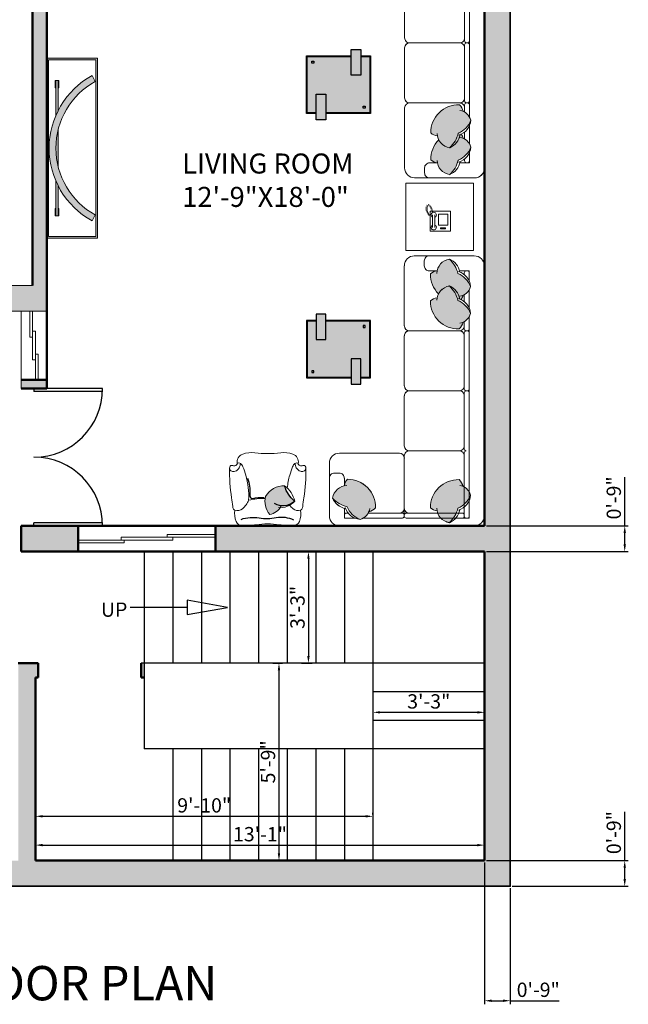
# Model space of a CAD drawing. Units: inches. Extents: x 1734 to 4011, y 1071 to 1891.
# Tile 15 of 27: x 3304 to 3517, y 1071 to 1415. Entities that reach past the tile are written whole.
import ezdxf

# ---------------------------------------------------------------- set-up
doc = ezdxf.new("R2010")
doc.units = ezdxf.units.IN
for name, color, linetype, lineweight in [('A-ANNO-DIMS', 2, 'Continuous', 18), ('A-ANNO-TEXT', 7, 'Continuous', 25), ('A-AREA-IDEN', 3, 'Continuous', 18), ('A-DOOR', 3, 'Continuous', 25), ('A-FLOR-STRS', 2, 'Continuous', 25), ('A-FURN', 8, 'Continuous', 18), ('A-FURN-PATT', 252, 'Continuous', 13), ('A-GLAZ', 4, 'Continuous', 18), ('A-WALL', 7, 'Continuous', 50), ('A-WALL-PATT', 8, 'Continuous', 13), ('aparador', 36, 'Continuous', 9), ('C-PROP', 1, 'Continuous', 35), ('moveis', 254, 'Continuous', 5)]:
    doc.layers.add(name, color=color, linetype=linetype, lineweight=lineweight)
doc.layers.add('IFF-FURN-DETAIL', color=250, linetype='Continuous')
doc.layers.add('MOBIL', color=7, linetype='Continuous')
doc.styles.get("Standard").update_dxf_attribs({"font": 'arial.ttf'})
doc.dimstyles.new('ISO-25', dxfattribs={"dimtxt": 5, "dimasz": 2.5, "dimexe": 1.25, "dimexo": 0.625, "dimtad": 1, "dimdec": 1, "dimlunit": 3, "dimtxsty": 'Standard', "dimcen": 2.5, "dimclrt": 1, "dimadec": 0, "dimazin": 0, "dimtfac": 1, "dimtdec": 1, "dimtmove": 0, "dimatfit": 3, "dimfxl": 1, "dimarcsym": 0})

# ---------------------------------------------------------------- blocks, each defined once
blk = doc.blocks.new('*D62')
at = {"layer": 'A-ANNO-DIMS', "color": 0, "lineweight": -2, "transparency": 16777216}
for p, q in [((3403.06, 1228.82), (3406.68, 1228.82)), ((3405.43, 1226.32), (3405.43, 1192.32)), ((3403.06, 1189.82), (3406.68, 1189.82))]:
    blk.add_line(p, q, dxfattribs=at)
at = {"layer": 'A-ANNO-DIMS', "color": 0, "transparency": 16777216}
for points in [[(3405.01, 1226.32), (3405.85, 1226.32), (3405.43, 1228.82)], [(3405.01, 1192.32), (3405.85, 1192.32), (3405.43, 1189.82)]]:
    blk.add_solid(points, dxfattribs=at)
at = {"layer": 'Defpoints', "color": 0, "transparency": 16777216}
for p in [(3402.43, 1228.82), (3402.43, 1189.82), (3405.43, 1189.82)]:
    blk.add_point(p, dxfattribs=at)
at = {"layer": 'A-ANNO-DIMS', "color": 0, "transparency": 16777216, "insert": (3402.25, 1209.32), "char_height": 5, "attachment_point": 5, "rotation": 90}
blk.add_mtext('3\'-3"', dxfattribs=at)
blk = doc.blocks.new('*D63')
at = {"layer": 'A-ANNO-DIMS', "color": 0, "lineweight": -2, "transparency": 16777216}
for p, q in [((3392.99, 1189.82), (3396.38, 1189.82)), ((3395.13, 1187.32), (3395.13, 1123.32)), ((3392.99, 1120.82), (3396.38, 1120.82))]:
    blk.add_line(p, q, dxfattribs=at)
at = {"layer": 'A-ANNO-DIMS', "color": 0, "transparency": 16777216}
for points in [[(3394.71, 1187.32), (3395.55, 1187.32), (3395.13, 1189.82)], [(3394.71, 1123.32), (3395.55, 1123.32), (3395.13, 1120.82)]]:
    blk.add_solid(points, dxfattribs=at)
at = {"layer": 'Defpoints', "color": 0, "transparency": 16777216}
for p in [(3392.36, 1189.82), (3392.36, 1120.82), (3395.13, 1120.82)]:
    blk.add_point(p, dxfattribs=at)
at = {"layer": 'A-ANNO-DIMS', "color": 0, "transparency": 16777216, "insert": (3391.95, 1155.32), "char_height": 5, "attachment_point": 5, "rotation": 90}
blk.add_mtext('5\'-9"', dxfattribs=at)
blk = doc.blocks.new('*D64')
at = {"layer": 'A-ANNO-DIMS', "color": 0, "lineweight": -2, "transparency": 16777216}
for p, q in [((3309.99, 1136.91), (3309.99, 1137.53)), ((3312.49, 1136.28), (3425.49, 1136.28)), ((3427.99, 1136.91), (3427.99, 1137.53))]:
    blk.add_line(p, q, dxfattribs=at)
at = {"layer": 'A-ANNO-DIMS', "color": 0, "transparency": 16777216}
for points in [[(3312.49, 1136.7), (3312.49, 1135.87), (3309.99, 1136.28)], [(3425.49, 1136.7), (3425.49, 1135.87), (3427.99, 1136.28)]]:
    blk.add_solid(points, dxfattribs=at)
at = {"layer": 'Defpoints', "color": 0, "transparency": 16777216}
for p in [(3309.99, 1136.28), (3427.99, 1136.28), (3427.99, 1136.28)]:
    blk.add_point(p, dxfattribs=at)
at = {"layer": 'A-ANNO-DIMS', "color": 0, "transparency": 16777216, "insert": (3368.99, 1139.46), "char_height": 5, "attachment_point": 5}
blk.add_mtext('9\'-10"', dxfattribs=at)
blk = doc.blocks.new('*D68')
at = {"layer": 'A-ANNO-DIMS', "color": 0, "lineweight": -2, "transparency": 16777216}
for p, q in [((3309.99, 1121.44), (3309.99, 1127.46)), ((3312.49, 1126.21), (3464.49, 1126.21)), ((3466.99, 1121.44), (3466.99, 1127.46))]:
    blk.add_line(p, q, dxfattribs=at)
at = {"layer": 'A-ANNO-DIMS', "color": 0, "transparency": 16777216}
for points in [[(3312.49, 1126.63), (3312.49, 1125.79), (3309.99, 1126.21)], [(3464.49, 1126.63), (3464.49, 1125.79), (3466.99, 1126.21)]]:
    blk.add_solid(points, dxfattribs=at)
at = {"layer": 'Defpoints', "color": 0, "transparency": 16777216}
for p in [(3466.99, 1126.21), (3309.99, 1120.82), (3466.99, 1120.82)]:
    blk.add_point(p, dxfattribs=at)
at = {"layer": 'A-ANNO-DIMS', "color": 0, "transparency": 16777216, "insert": (3388.49, 1129.39), "char_height": 5, "attachment_point": 5}
blk.add_mtext('13\'-1"', dxfattribs=at)
blk = doc.blocks.new('*D69')
at = {"layer": 'A-ANNO-DIMS', "color": 0, "lineweight": -2, "transparency": 16777216}
for p, q in [((3427.99, 1174.19), (3427.99, 1171.38)), ((3466.99, 1173.25), (3466.99, 1173.88)), ((3430.49, 1172.63), (3464.49, 1172.63))]:
    blk.add_line(p, q, dxfattribs=at)
at = {"layer": 'A-ANNO-DIMS', "color": 0, "transparency": 16777216}
for points in [[(3430.49, 1173.04), (3430.49, 1172.21), (3427.99, 1172.63)], [(3464.49, 1173.04), (3464.49, 1172.21), (3466.99, 1172.63)]]:
    blk.add_solid(points, dxfattribs=at)
at = {"layer": 'Defpoints', "color": 0, "transparency": 16777216}
for p in [(3427.99, 1174.82), (3466.99, 1172.63), (3466.99, 1172.63)]:
    blk.add_point(p, dxfattribs=at)
at = {"layer": 'A-ANNO-DIMS', "color": 0, "transparency": 16777216, "insert": (3447.49, 1175.8), "char_height": 5, "attachment_point": 5}
blk.add_mtext('3\'-3"', dxfattribs=at)
blk = doc.blocks.new("MD D 4'")
for p, q in [((0, 24), (0, 0)), ((1, 24), (1, 0)), ((47, 24), (47, 0)), ((48, 24), (48, 0)), ((0, 0), (1, 0)), ((48, 0), (47, 0))]:
    blk.add_line(p, q)
for centre, start, end in [((0, 0), 0, 90), ((48, 0), 90, 180)]:
    blk.add_arc(centre, 24, start, end)
blk = doc.blocks.new('Aparador ORGANICA Formatto')
at = {"layer": 'aparador', "ltscale": 0.3}
h = blk.add_hatch(color=256, dxfattribs=at)
h.dxf.hatch_style = 1
h.set_gradient(color1=(118, 213, 123), color2=(52, 168, 57), one_color=1, tint=0.43, name='INVCURVED')
h.paths.add_polyline_path([(0.8, 0.45), (-0.8, 0.45), (-0.8, 0), (0.8, 0)])
h.paths.add_polyline_path([(0.785, 0.435), (0.785, 0.015), (-0.785, 0.015), (-0.785, 0.435)], flags=16)
h.paths.add_polyline_path([(0.2911, 0.3699), (0.5365, 0.3699), (0.5365, 0.3757), (0.6011, 0.3757), (0.6011, 0.3699), (0.6011, 0.3499), (0.6011, 0.3441), (0.5365, 0.3441), (0.5365, 0.3499), (0.3338, 0.3499, -0.150336), (0.6449, 0.0488), (0.5923, 0.0199, 0.208852), (0.1632, 0.3499), (-0.1632, 0.3499, 0.208852), (-0.5923, 0.0199), (-0.6449, 0.0488, -0.150336), (-0.3338, 0.3499), (-0.5365, 0.3499), (-0.5365, 0.3441), (-0.6011, 0.3441), (-0.6011, 0.3499), (-0.6011, 0.3699), (-0.6011, 0.3757), (-0.5365, 0.3757), (-0.5365, 0.3699), (-0.2911, 0.3699, -0.206106)], flags=0)
h = blk.add_hatch(color=256, dxfattribs=at)
h.dxf.hatch_style = 1
h.set_gradient(color1=(135, 92, 69), color2=(0, 0, 0), one_color=1, name='INVCURVED')
h.paths.add_polyline_path([(-0.6449, 0.0488), (-0.5923, 0.0199, -0.590888), (0.5923, 0.0199), (0.6449, 0.0488, 0.590888)])
h = blk.add_hatch(color=256, dxfattribs=at)
h.dxf.hatch_style = 1
h.set_gradient(color1=(178, 189, 189), one_color=1, tint=1, name='CYLINDER')
h.paths.add_polyline_path([(-0.5365, 0.3757), (-0.6011, 0.3757), (-0.6011, 0.3699), (-0.5365, 0.3699)])
h.paths.add_polyline_path([(-0.5365, 0.3499), (-0.6011, 0.3499), (-0.6011, 0.3441), (-0.5365, 0.3441)])
h = blk.add_hatch(color=256, dxfattribs=at)
h.dxf.hatch_style = 1
h.set_gradient(color1=(118, 213, 123), color2=(31, 101, 35), one_color=1, tint=0.26, name='INVCURVED')
h.paths.add_polyline_path([(-0.2911, 0.3699), (-0.6011, 0.3699), (-0.6011, 0.3499), (-0.3338, 0.3499, -0.015999)])
h = blk.add_hatch(color=256, dxfattribs=at)
h.dxf.hatch_style = 1
h.set_gradient(color1=(118, 213, 123), color2=(31, 101, 35), one_color=1, tint=0.26, name='INVCURVED')
h.paths.add_polyline_path([(-0.1632, 0.3499), (0.1632, 0.3499, 0.122516)])
h = blk.add_hatch(color=256, dxfattribs=at)
h.dxf.hatch_style = 1
h.set_gradient(color1=(118, 213, 123), color2=(31, 101, 35), one_color=1, tint=0.26, name='INVCURVED')
h.paths.add_polyline_path([(0.6011, 0.3699), (0.2911, 0.3699, -0.015999), (0.3338, 0.3499), (0.6011, 0.3499)])
h = blk.add_hatch(color=256, dxfattribs=at)
h.dxf.hatch_style = 1
h.set_gradient(color1=(178, 189, 189), one_color=1, tint=1, name='CYLINDER')
h.paths.add_polyline_path([(0.6011, 0.3757), (0.5365, 0.3757), (0.5365, 0.3699), (0.6011, 0.3699)])
h.paths.add_polyline_path([(0.6011, 0.3499), (0.5365, 0.3499), (0.5365, 0.3441), (0.6011, 0.3441)])
for p, q in [((-0.5923, 0.0199), (-0.6449, 0.0488)), ((0.5923, 0.0199), (0.6449, 0.0488))]:
    blk.add_line(p, q, dxfattribs=at)
for points in [[(-0.6011, 0.3699), (-0.6011, 0.3757), (-0.5365, 0.3757), (-0.5365, 0.3699)], [(-0.5365, 0.3499), (-0.5365, 0.3441), (-0.6011, 0.3441), (-0.6011, 0.3499)], [(0.6011, 0.3699), (0.6011, 0.3757), (0.5365, 0.3757), (0.5365, 0.3699)], [(0.5365, 0.3499), (0.5365, 0.3441), (0.6011, 0.3441), (0.6011, 0.3499)]]:
    blk.add_lwpolyline(points, dxfattribs=at)
for radius in [0.7362, 0.6762]:
    blk.add_arc((0, -0.3063), radius, 28.84335, 151.15665, dxfattribs=at)
at = {"layer": 'moveis', "ltscale": 0.3}
for p, q in [((-0.6011, 0.3699), (-0.6011, 0.3499)), ((-0.2911, 0.3699), (-0.6011, 0.3699)), ((-0.6011, 0.3499), (-0.3338, 0.3499)), ((-0.1632, 0.3499), (0.1632, 0.3499)), ((0.2911, 0.3699), (0.6011, 0.3699)), ((0.6011, 0.3499), (0.3338, 0.3499)), ((0.6011, 0.3699), (0.6011, 0.3499))]:
    blk.add_line(p, q, dxfattribs=at)
for points in [[(-0.8, 0), (0.8, 0), (0.8, 0.45), (-0.8, 0.45)], [(-0.785, 0.015), (0.785, 0.015), (0.785, 0.435), (-0.785, 0.435)]]:
    blk.add_lwpolyline(points, close=True, dxfattribs=at)
blk = doc.blocks.new('Mesa de centro Cantria feeling')
at = {"layer": 'MOBIL', "ltscale": 0.2}
h = blk.add_hatch(color=256, dxfattribs=at)
h.set_gradient(color1=(74, 55, 38), color2=(104, 77, 54), one_color=1, tint=0.31, name='CYLINDER')
h.paths.add_polyline_path([(-0.85, -0.3), (-0.7, -0.3), (-0.7, 0.1), (-0.85, 0.1)])
h = blk.add_hatch(color=256, dxfattribs=at)
h.set_gradient(color1=(221, 221, 223), one_color=1, tint=1)
h.paths.add_polyline_path([(-0.15, -0.6), (-0.15, -0.89), (-0.01, -0.89), (-0.01, -0.01), (-0.7, -0.01), (-0.7, -0.3), (-0.85, -0.3), (-0.85, -0.01), (-0.99, -0.01), (-0.99, -0.89), (-0.3, -0.89), (-0.3, -0.6)])
h.paths.add_polyline_path([(-0.112, -0.112), (-0.112, -0.082), (-0.082, -0.082), (-0.082, -0.112)], flags=16)
h.paths.add_polyline_path([(-0.888, -0.788), (-0.888, -0.818), (-0.918, -0.818), (-0.918, -0.788)], flags=16)
h = blk.add_hatch(color=256, dxfattribs=at)
h.set_gradient(color1=(74, 55, 38), color2=(104, 77, 54), one_color=1, tint=0.31, name='CYLINDER')
h.paths.add_polyline_path([(-0.15, -0.6), (-0.3, -0.6), (-0.3, -1), (-0.15, -1)])
for points in [[(-0.85, 0), (-1, 0), (-1, -0.9), (-0.3, -0.9)], [(-0.15, -0.9), (0, -0.9), (0, 0), (-0.7, 0)], [(-0.85, -0.01), (-0.99, -0.01), (-0.99, -0.89), (-0.3, -0.89)], [(-0.15, -0.89), (-0.01, -0.89), (-0.01, -0.01), (-0.7, -0.01)]]:
    blk.add_lwpolyline(points, dxfattribs=at)
for points in [[(-0.85, -0.3), (-0.7, -0.3), (-0.7, 0.1), (-0.85, 0.1)], [(-0.082, -0.082), (-0.112, -0.082), (-0.112, -0.112), (-0.082, -0.112)], [(-0.15, -0.6), (-0.3, -0.6), (-0.3, -1), (-0.15, -1)], [(-0.918, -0.818), (-0.888, -0.818), (-0.888, -0.788), (-0.918, -0.788)]]:
    blk.add_lwpolyline(points, close=True, dxfattribs=at)
blk = doc.blocks.new('SOFA 1')
at = {"transparency": 33554687}
h = blk.add_hatch(color=256, dxfattribs=at)
h.dxf.hatch_style = 1
h.paths.add_polyline_path([(3769.65, 1307.6, 0.084911), (3767.15, 1309.12, 0.046133), (3766.46, 1311.13), (3759.18, 1311.13, 0.039409), (3758.92, 1310.24, 0.165523), (3756.31, 1309.02, 0.42585), (3767.59, 1297.95, 0.121928), (3769.15, 1300.58, 0.027403), (3769.65, 1300.83)])
h.paths.add_polyline_path([(3765.34, 1313.08), (3760.4, 1313.08, 0.097704), (3759.18, 1311.13), (3766.46, 1311.13, 0.04873)])
h.paths.add_polyline_path([(3763.76, 1314.88, 0.16488), (3760.4, 1313.08), (3765.34, 1313.08, 0.051917)])
h.paths.add_polyline_path([(3771.6, 1305.17, 0.090388), (3769.65, 1307.6), (3769.65, 1300.83, 0.136035), (3771.6, 1302.77)])
h = blk.add_hatch(color=256, dxfattribs=at)
h.dxf.hatch_style = 1
h.paths.add_polyline_path([(3723.52, 1308.63, 0.147724), (3717.76, 1305.24, 0.310469), (3722.42, 1300.4), (3722.42, 1300.25, 0.156703), (3723.62, 1297.8, 0.425821), (3734.69, 1309.08, 0.121928), (3732.05, 1310.63, 0.233216), (3728.6, 1313.59, 0.213835)])
h = blk.add_hatch(color=256, dxfattribs=at)
h.dxf.hatch_style = 1
h.paths.add_polyline_path([(3769.16, 1235.96, 0.122267), (3767.6, 1238.61, 0.425972), (3756.32, 1227.54, 0.165563), (3758.93, 1226.32, 0.309481), (3763.76, 1221.69, 0.002677), (3763.83, 1221.72, 0.146094), (3767.16, 1227.43, 0.212433), (3772.1, 1232.48, 0.235342)])
h = blk.add_hatch(color=256, dxfattribs=at)
h.dxf.hatch_style = 1
h.paths.add_polyline_path([(3769.16, 1225.36, 0.122267), (3767.6, 1228.01, 0.425972), (3756.32, 1216.94, 0.165563), (3758.93, 1215.72, 0.309481), (3763.76, 1211.09, 0.002677), (3763.83, 1211.12, 0.146094), (3767.16, 1216.83, 0.212433), (3772.1, 1221.88, 0.235342)])
for p, q in [((3720.45, 1316.13), (3773.58, 1316.13)), ((3777.51, 1312.19), (3777.51, 1213.72))]:
    blk.add_line(p, q, dxfattribs=at)
for points in [[(3763.76, 1314.88, -0.147724), (3767.15, 1309.12, -0.213355), (3772.1, 1304.05, 0.213355), (3767.15, 1309.12, 0.147724), (3763.76, 1314.88, -0.249545), (3767.86, 1309.77, 0.249545), (3763.77, 1314.89, 0.356779), (3758.8, 1309.23, -0.356779), (3763.76, 1314.88)], [(3717.76, 1305.24, -0.147724), (3723.52, 1308.63, -0.213355), (3728.59, 1313.59, 0.213355), (3723.52, 1308.63, 0.147724), (3717.76, 1305.24, -0.249545), (3722.86, 1309.34, 0.249545), (3717.75, 1305.25, 0.356779), (3723.4, 1300.28, -0.356779), (3717.76, 1305.24)], [(3734.69, 1309.08, -0.425972), (3723.62, 1297.8, -0.165552), (3722.4, 1300.4, 0.165552), (3723.62, 1297.79, 0.425972), (3734.69, 1309.07, 0.121514), (3732.07, 1310.63, -0.121514), (3734.69, 1309.08)], [(3728.58, 1313.6, -0.306333), (3732.42, 1309.31, 0.306333), (3728.58, 1313.6, 0.306674), (3722.72, 1308.89, -0.306674), (3728.58, 1313.6)], [(3767.6, 1297.95, -0.425972), (3756.31, 1309.01, -0.165552), (3758.92, 1310.24, 0.165552), (3756.31, 1309.02, 0.425972), (3767.59, 1297.95, 0.121514), (3769.14, 1300.57, -0.121514), (3767.6, 1297.95)], [(3772.11, 1304.06, -0.306333), (3767.83, 1300.22, 0.306333), (3772.11, 1304.06, 0.306674), (3767.4, 1309.91, -0.306674), (3772.11, 1304.06)], [(3770.44, 1286.63, -0.414214), (3769.66, 1287.4, 0.414214), (3770.44, 1286.63, 0.414214), (3769.66, 1285.83, -0.414214), (3770.44, 1286.63)], [(3748.01, 1262.99, -0.414214), (3746.05, 1264.95, 0.414214), (3748.01, 1262.97, 0.414213), (3746.05, 1261.01, -0.414213), (3748.01, 1262.99)], [(3770.44, 1262.99, -0.414214), (3769.66, 1263.77, 0.414214), (3770.44, 1262.99, 0.414214), (3769.66, 1262.19, -0.414214), (3770.44, 1262.99)], [(3770.83, 1262.97, -0.414214), (3771.61, 1262.19, 0.414214), (3770.83, 1262.99, 0.414214), (3771.61, 1263.77, -0.414214), (3770.83, 1262.97)], [(3748.01, 1239.35, -0.414214), (3746.05, 1241.31, 0.414214), (3748.01, 1239.33, 0.414213), (3746.05, 1237.37, -0.414213), (3748.01, 1239.35)], [(3767.7, 1239.33, -0.414214), (3769.66, 1237.37, 0.414214), (3767.7, 1239.35, 0.414214), (3769.66, 1241.31, -0.414214), (3767.7, 1239.33)], [(3756.32, 1227.54, -0.425972), (3767.6, 1238.61, -0.121514), (3769.16, 1235.98, 0.121514), (3767.6, 1238.61, 0.425972), (3756.32, 1227.54, 0.165552), (3758.93, 1226.32, -0.165552), (3756.32, 1227.54)], [(3770.44, 1239.35, -0.414214), (3769.66, 1240.13, 0.414214), (3770.44, 1239.33, 0.414214), (3769.66, 1238.55, -0.414214), (3770.44, 1239.35)], [(3770.83, 1239.33, -0.414214), (3771.61, 1238.55, 0.414214), (3770.83, 1239.35, 0.414214), (3771.61, 1240.13, -0.414214), (3770.83, 1239.33)], [(3772.1, 1232.5, -0.306674), (3767.41, 1226.64, 0.306674), (3772.1, 1232.5, 0.306333), (3767.84, 1236.34, -0.306333), (3772.1, 1232.5)], [(3763.78, 1221.67, 0.249545), (3767.87, 1226.78, -0.249545), (3763.76, 1221.69, -0.356779), (3758.81, 1227.32, 0.356779), (3763.77, 1221.68, 0.147724), (3767.16, 1227.43, 0.213355), (3772.11, 1232.51, -0.213355), (3767.16, 1227.43, -0.147724), (3763.78, 1221.67)], [(3756.32, 1216.94, -0.200233), (3759.49, 1224.76, 0.200233), (3756.32, 1216.94, 0.165552), (3758.93, 1215.72, -0.165552), (3756.32, 1216.94)], [(3772.1, 1221.9, -0.306674), (3767.41, 1216.04, 0.306674), (3772.1, 1221.9, -0.213355), (3767.16, 1216.83, -0.147724), (3763.77, 1211.08, 0.147724), (3767.15, 1216.83, 0.213355), (3772.1, 1221.9)], [(3763.76, 1211.09, -0.356779), (3758.81, 1216.72, 0.356779), (3763.76, 1211.09, 0.249545), (3767.87, 1216.18, -0.249545), (3763.76, 1211.09)]]:
    blk.add_lwpolyline(points, format="xyb", dxfattribs=at)
for points in [[(3716.51, 1312.2), (3716.51, 1291.44)], [(3722.42, 1313.08), (3722.42, 1309.23), (3722.42, 1313.08), (3726.57, 1313.08)], [(3723.21, 1311.13), (3723.93, 1311.13)], [(3729.85, 1313.08), (3745.25, 1313.08)], [(3731.82, 1311.13), (3745.25, 1311.13)], [(3746.01, 1312.3), (3746.01, 1288.55)], [(3746.01, 1310.97), (3746.01, 1311.36)], [(3768.11, 1313.08), (3746.78, 1313.08)], [(3768.87, 1311.13), (3746.78, 1311.13)], [(3771.6, 1313.08), (3767.75, 1313.08), (3771.6, 1313.08), (3771.6, 1308.93)], [(3769.66, 1287.39), (3769.65, 1312.3)], [(3771.6, 1313.08), (3771.61, 1233.74)], [(3746.01, 1288.54), (3746.01, 1308.23)], [(3769.65, 1309.43), (3769.65, 1308.71)], [(3722.42, 1300.39), (3722.42, 1297.33)], [(3720.45, 1295.38), (3718.48, 1295.38)], [(3720.45, 1287.5), (3744.09, 1287.5)], [(3746.02, 1284.63), (3746.02, 1264.94)], [(3747.99, 1286.6), (3767.69, 1286.6)], [(3769.66, 1263.75), (3769.66, 1285.81)], [(3769.66, 1277.18), (3769.66, 1263.75)], [(3746.02, 1260.99), (3746.02, 1241.3)], [(3747.99, 1262.97), (3767.69, 1262.97)], [(3769.66, 1240.12), (3769.66, 1262.18)], [(3770.43, 1262.97), (3770.82, 1262.97)], [(3746.02, 1237.36), (3746.02, 1213.74)], [(3747.99, 1239.33), (3767.69, 1239.33)], [(3769.66, 1235.71), (3769.66, 1238.54)], [(3770.43, 1239.33), (3770.82, 1239.33)], [(3771.61, 1223.14), (3771.61, 1230.47)], [(3769.66, 1225.11), (3769.66, 1227.82)], [(3767.76, 1215.72), (3771.61, 1215.72), (3771.61, 1219.84), (3771.61, 1215.72)], [(3753.91, 1211.77), (3753.91, 1213.74)], [(3755.86, 1215.72), (3758.92, 1215.72)], [(3769.66, 1216.5), (3769.66, 1217.22)], [(3749.97, 1209.8), (3773.58, 1209.8)]]:
    blk.add_lwpolyline(points, close=True, dxfattribs=at)
for points in [[(3722.42, 1311.91, 0.414214), (3723.2, 1311.13, -0.414214)], [(3770.43, 1313.08, 0.414214), (3769.65, 1312.3, -0.414214)], [(3771.6, 1312.3, 0.414214), (3770.82, 1313.08, -0.414214)], [(3716.51, 1297.34, 0.414214), (3718.47, 1295.38, -0.414214)], [(3720.44, 1295.38, 0.414214), (3722.4, 1297.34, -0.414214)], [(3716.51, 1291.45, 0.414212), (3720.44, 1287.52, -0.414212)], [(3746.03, 1288.56, 0.414214), (3747.99, 1286.6, 0.414213), (3746.03, 1284.64, -0.414213), (3747.99, 1286.6, -0.414214)], [(3769.66, 1284.64, 0.414214), (3767.7, 1286.6, 0.414214), (3769.66, 1288.56, -0.414214), (3767.7, 1286.6, -0.414214)], [(3769.66, 1261.01, 0.414214), (3767.7, 1262.97, 0.414214), (3769.66, 1264.93, -0.414214), (3767.7, 1262.97, -0.414214)], [(3772.13, 1221.9, 0.306333), (3767.84, 1225.74, -0.306333)], [(3769.16, 1225.36, 0.071861), (3768.39, 1227.01, -0.071861)], [(3746.05, 1213.76, 0.414212), (3749.98, 1209.82, -0.414212)], [(3755.87, 1215.72, 0.414214), (3753.91, 1213.76, -0.414214)], [(3769.66, 1216.52, 0.414214), (3770.44, 1215.74, -0.414214)], [(3770.83, 1215.74, 0.414214), (3771.61, 1216.52, -0.414214)], [(3755.87, 1209.8, -0.414214), (3753.91, 1211.76, 0.414214)]]:
    blk.add_lwpolyline(points, format="xyb", close=True, dxfattribs=at)
for centre, radius, start, end in [((3720.44, 1312.2), 3.93, 90.0002, 179.9998), ((3720.44, 1312.19), 3.94, 89.9158, 179.9154), ((3773.58, 1312.2), 3.93, 0.0002, 89.9998), ((3773.57, 1312.19), 3.94, 359.9158, 89.9154), ((3744.09, 1309.21), 1.92, 358.766, 90.5111), ((3745.22, 1312.29), 0.789, 0.8425, 90.8425), ((3745.24, 1311.91), 0.777, 270, 0), ((3745.24, 1311.91), 0.777, 270, 0), ((3746.8, 1312.29), 0.789, 89.1575, 179.1575), ((3746.79, 1311.91), 0.777, 180, 270), ((3746.79, 1311.91), 0.777, 180, 270), ((3747.93, 1309.21), 1.92, 89.4889, 181.234), ((3768.87, 1312.3), 0.777, 360, 90), ((3768.87, 1311.91), 0.777, 270, 0), ((3744.08, 1289.48), 1.96, 270, 360), ((3744.08, 1289.48), 1.96, 270, 360), ((3773.58, 1213.73), 3.93, 270.0002, 359.9998), ((3773.59, 1213.73), 3.93, 269.9156, 359.9152)]:
    blk.add_arc(centre, radius, start, end, dxfattribs=at)
blk = doc.blocks.new('PILLOW-1')
at = {"color": 0}
blk.add_lwpolyline([(198, -165, -0.232884), (126, -346, -0.184752), (-44, -234, -0.286563), (75, -22, -0.237978), (273, -68, -0.243587), (179, -195, 4.263709)], format="xyb", dxfattribs=at)
at = {"layer": 'IFF-FURN-DETAIL'}
blk.add_lwpolyline([(148, -118, -0.343333), (126, -342, 0.126408), (-40, -233, -5.969376)], format="xyb", dxfattribs=at)
blk = doc.blocks.new('CLNG90')
for points in [[(689, 370, 0.157831), (677, 385, 0.121013), (646, 395, -0.017334), (547, 407, 0.041496), (215, 431, 0.153531), (191, 423, 0.382906), (185, 395, -0.284047), (184, 361, 0.011997), (177, 351, -0.370479), (160, 345, 0.380647), (56, 282, 0.117468), (41, 146, -0.027775), (50, 0, -8.773898)], [(160, 345, 0.22481), (160, 306, 0.055398), (209, 322, 0.180116), (249, 368, 0.194833), (248, 405, 0.242377), (215, 431, 1.52074)], [(160, 345, 0.22481), (160, 306, 0.055398), (209, 322, 0.180116), (249, 368, 0.194833), (248, 405, 0.242377), (215, 431, 1.52074)], [(689, 370, -0.235486), (671, 286, -0.134038), (574, 215, -0.079303), (293, 248, -0.027048), (199, 280, -0.106276), (160, 306, -1.699)], [(689, 370, -0.235486), (671, 286, -0.134038), (574, 215, -0.079303), (293, 248, -0.027048), (199, 280, -0.106276), (160, 306, -1.699)], [(689, 370, -0.146607), (814, 357, -0.305296), (862, 286, -0.042137), (852, 131, 0.040285), (843, 0, 3.952121)], [(574, 215, 0.061244), (556, 29, 3.376255)], [(574, 215, 0.061244), (556, 29, 3.376255)], [(689, -370, -0.157831), (677, -385, -0.121013), (646, -395, 0.017334), (547, -407, -0.041496), (215, -431, -0.153531), (191, -423, -0.382906), (185, -395, 0.284047), (184, -361, -0.011997), (177, -351, 0.370479), (160, -345, -0.380647), (56, -282, -0.117468), (41, -146, 0.027775), (50, 0, 8.773898)], [(689, -370, 0.146607), (814, -357, 0.305296), (862, -286, 0.042137), (852, -131, -0.040285), (843, 0, -3.952121)], [(437, -220, 0.041086), (293, -248, 0.027048), (199, -280, 0.106276), (160, -306, 1.699)], [(437, -220, 0.041086), (293, -248, 0.027048), (199, -280, 0.106276), (160, -306, 1.699)], [(160, -345, -0.22481), (160, -306, -0.055398), (209, -322, -0.180116), (249, -368, -0.194833), (248, -405, -0.242377), (215, -431, -1.52074)], [(160, -345, -0.22481), (160, -306, -0.055398), (209, -322, -0.180116), (249, -368, -0.194833), (248, -405, -0.242377), (215, -431, -1.52074)], [(689, -370, 0.235486), (671, -286, 0.060693), (632, -247, 0.001296)], [(689, -370, 0.235486), (671, -286, 0.060693), (632, -247, 0.001296)]]:
    blk.add_lwpolyline(points, format="xyb")
at = {"layer": 'IFF-FURN-DETAIL'}
for points in [[(328, 228, 0.109125), (508, 203, -0.16587), (546, 194, -0.314359), (555, 172, 0.072017), (544, 42, 4.351186)], [(328, 228, 0.109125), (508, 203, -0.16587), (546, 194, -0.314359), (555, 172, 0.072017), (544, 42, 4.351186)], [(791, 301, 0.124986), (774, 96, -0.091334), (771, -95, 0.164688), (797, -292, 1.068868)], [(791, 301, 0.124986), (774, 96, -0.091334), (771, -95, 0.164688), (797, -292, 1.068868)]]:
    blk.add_lwpolyline(points, format="xyb", dxfattribs=at)
at = {"xscale": 1.016, "yscale": 1.016, "zscale": 1.016}
blk.add_blockref('PILLOW-1', (458, 47), dxfattribs=at)
blk.add_blockref('PILLOW-1', (458, 47), dxfattribs=at)
blk = doc.blocks.new('*D124')
at = {"layer": 'A-ANNO-DIMS', "color": 0, "lineweight": -2, "transparency": 16777216}
for p, q in [((3515.99, 1120.82), (3515.99, 1137.86)), ((3467.62, 1120.82), (3517.24, 1120.82)), ((3515.99, 1114.32), (3515.99, 1118.32)), ((3476.62, 1111.82), (3517.24, 1111.82))]:
    blk.add_line(p, q, dxfattribs=at)
at = {"layer": 'A-ANNO-DIMS', "color": 0, "transparency": 16777216}
for points in [[(3515.58, 1118.32), (3516.41, 1118.32), (3515.99, 1120.82)], [(3515.58, 1114.32), (3516.41, 1114.32), (3515.99, 1111.82)]]:
    blk.add_solid(points, dxfattribs=at)
at = {"layer": 'Defpoints', "color": 0, "transparency": 16777216}
for p in [(3466.99, 1120.82), (3515.99, 1120.82), (3475.99, 1111.82)]:
    blk.add_point(p, dxfattribs=at)
at = {"layer": 'A-ANNO-DIMS', "color": 1, "transparency": 16777216, "insert": (3512.82, 1130.59), "char_height": 5, "attachment_point": 5, "rotation": 90}
blk.add_mtext('0\'-9"', dxfattribs=at)
blk = doc.blocks.new('*D125')
at = {"layer": 'A-ANNO-DIMS', "color": 0, "lineweight": -2, "transparency": 16777216}
for p, q in [((3515.99, 1237.82), (3515.99, 1254.86)), ((3467.62, 1237.82), (3517.24, 1237.82)), ((3515.99, 1231.32), (3515.99, 1235.32)), ((3467.62, 1228.82), (3517.24, 1228.82))]:
    blk.add_line(p, q, dxfattribs=at)
at = {"layer": 'A-ANNO-DIMS', "color": 0, "transparency": 16777216}
for points in [[(3515.58, 1235.32), (3516.41, 1235.32), (3515.99, 1237.82)], [(3515.58, 1231.32), (3516.41, 1231.32), (3515.99, 1228.82)]]:
    blk.add_solid(points, dxfattribs=at)
at = {"layer": 'Defpoints', "color": 0, "transparency": 16777216}
for p in [(3466.99, 1237.82), (3515.99, 1237.82), (3466.99, 1228.82)]:
    blk.add_point(p, dxfattribs=at)
at = {"layer": 'A-ANNO-DIMS', "color": 1, "transparency": 16777216, "insert": (3512.82, 1247.59), "char_height": 5, "attachment_point": 5, "rotation": 90}
blk.add_mtext('0\'-9"', dxfattribs=at)
blk = doc.blocks.new('*D126')
at = {"layer": 'A-ANNO-DIMS', "color": 0, "lineweight": -2, "transparency": 16777216}
for p, q in [((3466.99, 1120.19), (3466.99, 1070.57)), ((3475.99, 1111.19), (3475.99, 1070.57)), ((3469.49, 1071.82), (3473.49, 1071.82)), ((3475.99, 1071.82), (3493.03, 1071.82))]:
    blk.add_line(p, q, dxfattribs=at)
at = {"layer": 'A-ANNO-DIMS', "color": 0, "transparency": 16777216}
for points in [[(3469.49, 1072.24), (3469.49, 1071.4), (3466.99, 1071.82)], [(3473.49, 1072.24), (3473.49, 1071.4), (3475.99, 1071.82)]]:
    blk.add_solid(points, dxfattribs=at)
at = {"layer": 'Defpoints', "color": 0, "transparency": 16777216}
for p in [(3466.99, 1120.82), (3475.99, 1111.82), (3475.99, 1071.82)]:
    blk.add_point(p, dxfattribs=at)
at = {"layer": 'A-ANNO-DIMS', "color": 1, "transparency": 16777216, "insert": (3485.76, 1075), "char_height": 5, "attachment_point": 5}
blk.add_mtext('0\'-9"', dxfattribs=at)

msp = doc.modelspace()

# ---------------------------------------------------------------- hatches: boundary and pattern name
at = {"layer": 'A-FURN-PATT'}
h = msp.add_hatch(color=256, dxfattribs=at)
h.dxf.hatch_style = 1
h.paths.add_polyline_path([(3390.43, 1248.05, 0.237978), (3391.88, 1241.82, 0.250405), (3395.95, 1244.88, 0.218011), (3400.51, 1246.42, -0.129718), (3397.01, 1251.81, 0.283254)])
at = {"layer": 'A-WALL-PATT'}
h = msp.add_hatch(color=256, dxfattribs=at)
h.dxf.hatch_style = 1
h.paths.add_polyline_path([(3475.99, 1831.82), (3115.99, 1831.82), (3115.99, 1745.82), (3130.99, 1745.82), (3130.99, 1750.82), (3124.99, 1750.82), (3124.99, 1822.82), (3214.99, 1822.82), (3214.99, 1780.82), (3219.99, 1780.82), (3219.99, 1822.82), (3308.99, 1822.82), (3308.99, 1750.82), (3254.99, 1750.82), (3254.99, 1745.82), (3308.99, 1745.82), (3308.99, 1604.82), (3313.99, 1604.82), (3313.99, 1745.82), (3366.99, 1745.82), (3366.99, 1750.82), (3313.99, 1750.82), (3313.99, 1822.82), (3401.99, 1822.82), (3401.99, 1750.82), (3396.99, 1750.82), (3396.99, 1745.82), (3411.99, 1745.82), (3411.99, 1750.82), (3406.99, 1750.82), (3406.99, 1822.82), (3466.99, 1822.82), (3466.99, 1750.82), (3441.99, 1750.82), (3441.99, 1745.82), (3466.99, 1745.82), (3466.99, 1517.82), (3452.49, 1517.82), (3452.49, 1512.82), (3466.99, 1512.82), (3466.99, 1458.82), (3446.49, 1458.82), (3446.49, 1453.82), (3466.99, 1453.82), (3466.99, 1237.82), (3372.99, 1237.82), (3372.99, 1228.82), (3466.99, 1228.82), (3466.99, 1120.82), (3309.99, 1120.82), (3309.99, 1184.82), (3310.99, 1184.82), (3310.99, 1189.82), (3303.99, 1189.82), (3303.99, 1120.82), (3291.99, 1120.82), (3291.99, 1111.82), (3475.99, 1111.82)])
h.paths.add_polyline_path([(3169.99, 1745.82), (3224.99, 1745.82), (3224.99, 1750.82), (3154.99, 1750.82), (3154.99, 1745.82), (3160.99, 1745.82), (3160.99, 1636.82), (3169.99, 1636.82)], flags=17)
h.paths.add_polyline_path([(3169.99, 1588.82), (3160.99, 1588.82), (3160.99, 1559.82), (3313.99, 1559.82), (3313.99, 1568.82), (3308.99, 1568.82), (3308.99, 1564.82), (3169.99, 1564.82)], flags=17)
h.paths.add_polyline_path([(3416.49, 1517.82), (3401.99, 1517.82), (3401.99, 1512.82), (3416.49, 1512.82)], flags=17)
h.paths.add_polyline_path([(3371.99, 1517.82), (3366.99, 1517.82), (3366.99, 1453.82), (3392.49, 1453.82), (3392.49, 1458.82), (3371.99, 1458.82)], flags=17)
h.paths.add_polyline_path([(3258.99, 1529.82), (3160.99, 1529.82), (3160.99, 1494.82), (3169.99, 1494.82), (3169.99, 1524.82), (3253.99, 1524.82), (3253.99, 1520.82), (3258.99, 1520.82)], flags=17)
h.paths.add_polyline_path([(3263.99, 1458.82), (3258.99, 1458.82), (3258.99, 1490.82), (3253.99, 1490.82), (3253.99, 1458.82), (3169.99, 1458.82), (3169.99, 1470.82), (3160.99, 1470.82), (3160.99, 1387.82), (3169.99, 1387.82), (3169.99, 1453.82), (3263.99, 1453.82)], flags=17)
h.paths.add_polyline_path([(3313.99, 1453.82), (3318.99, 1453.82), (3318.99, 1458.82), (3299.99, 1458.82), (3299.99, 1453.82), (3308.99, 1453.82), (3308.99, 1321.82), (3266.49, 1321.82), (3266.49, 1312.82), (3313.99, 1312.82)], flags=17)
h.paths.add_polyline_path([(3212.49, 1321.82), (3169.99, 1321.82), (3169.99, 1339.82), (3160.99, 1339.82), (3160.99, 1312.82), (3212.49, 1312.82)], flags=17)
h.paths.add_polyline_path([(3313.99, 1288.82), (3304.99, 1288.82), (3304.99, 1285.82), (3313.99, 1285.82)], flags=17)
h.paths.add_polyline_path([(3324.99, 1237.82), (3304.99, 1237.82), (3304.99, 1228.82), (3324.99, 1228.82)], flags=17)
h = msp.add_hatch(color=256, dxfattribs=at)
h.dxf.hatch_style = 1
h.paths.add_polyline_path([(3347.99, 1189.82), (3346.99, 1189.82), (3346.99, 1184.82), (3347.99, 1184.82)])

# ---------------------------------------------------------------- linework, layer by layer
at = {"layer": 'A-FLOR-STRS'}
for p, q in [((3347.99, 1228.82), (3347.99, 1159.82)), ((3357.99, 1228.82), (3357.99, 1189.82)), ((3367.99, 1228.82), (3367.99, 1189.82)), ((3377.99, 1228.82), (3377.99, 1189.82)), ((3387.99, 1228.82), (3387.99, 1189.82)), ((3397.99, 1228.82), (3397.99, 1189.82)), ((3407.99, 1228.82), (3407.99, 1189.82)), ((3417.99, 1228.82), (3417.99, 1189.82)), ((3427.99, 1228.82), (3427.99, 1120.82)), ((3362.99, 1209.32), (3343.07, 1209.32)), ((3466.99, 1189.82), (3346.99, 1189.82)), ((3466.99, 1179.82), (3427.99, 1179.82)), ((3466.99, 1169.82), (3427.99, 1169.82)), ((3466.99, 1159.82), (3347.99, 1159.82)), ((3357.99, 1159.82), (3357.99, 1120.82)), ((3367.99, 1159.82), (3367.99, 1120.82)), ((3377.99, 1159.82), (3377.99, 1120.82)), ((3387.99, 1159.82), (3387.99, 1120.82)), ((3397.99, 1159.82), (3397.99, 1120.82)), ((3407.99, 1159.82), (3407.99, 1120.82)), ((3417.99, 1159.82), (3417.99, 1120.82))]:
    msp.add_line(p, q, dxfattribs=at)
msp.add_lwpolyline([(3377.15, 1209.32), (3362.99, 1211.87), (3362.99, 1206.77)], close=True, dxfattribs=at)
at = {"layer": 'A-FURN'}
for p, q in [((3169.99, 1321.82), (3308.99, 1321.82)), ((3124.99, 1312.82), (3313.99, 1312.82)), ((3304.99, 1312.82), (3304.99, 1285.82))]:
    msp.add_line(p, q, dxfattribs=at)
for points in [[(3439.5, 1334.01), (3439.5, 1357.63), (3463.12, 1357.63), (3463.12, 1334.01)], [(3446.69, 1349.53), (3447.2, 1349.37)], [(3447.74, 1349.72), (3448.25, 1349.53)], [(3447.04, 1347.12), (3447.55, 1346.93)], [(3447.99, 1347.81), (3455.09, 1347.81), (3455.09, 1340.81), (3447.99, 1340.81)], [(3455.09, 1347.81), (3455.09, 1340.81), (3447.99, 1340.81), (3447.99, 1347.81)], [(3448.78, 1346.49), (3448.78, 1342.15)], [(3449.64, 1346.49), (3449.64, 1342.15)], [(3454.16, 1342.94), (3450.91, 1342.94), (3450.91, 1346.75), (3454.16, 1346.75)], [(3450.91, 1342.94), (3450.91, 1346.75), (3454.16, 1346.75), (3454.16, 1342.94)], [(3453.35, 1341.99), (3453.35, 1341.6), (3451.61, 1341.6), (3451.61, 1341.99)], [(3451.61, 1341.99), (3453.35, 1341.99), (3453.35, 1341.6), (3451.61, 1341.6)]]:
    msp.add_lwpolyline(points, close=True, dxfattribs=at)
msp.add_lwpolyline([(3463.12, 1357.63), (3463.12, 1334.01), (3439.5, 1334.01), (3439.5, 1357.63)], dxfattribs=at)
for points in [[(3449.67, 1345.7, 3.938511), (3448.8, 1345.7, -3.938511)], [(3448.8, 1342.97, 3.938511), (3449.67, 1342.97, -3.938511)]]:
    msp.add_lwpolyline(points, format="xyb", close=True, dxfattribs=at)
at = {"layer": 'A-GLAZ'}
for p, q in [((3307.99, 1303.82), (3307.99, 1312.82)), ((3308.99, 1295.82), (3308.99, 1312.82)), ((3309.99, 1305.82), (3308.99, 1305.82)), ((3309.99, 1288.82), (3309.99, 1305.82)), ((3308.99, 1303.82), (3307.99, 1303.82)), ((3310.99, 1297.82), (3309.99, 1297.82)), ((3310.99, 1288.82), (3310.99, 1297.82)), ((3309.99, 1295.82), (3308.99, 1295.82)), ((3324.99, 1232.82), (3357.99, 1232.82)), ((3339.99, 1233.82), (3372.99, 1233.82)), ((3339.99, 1232.82), (3339.99, 1233.82)), ((3340.99, 1231.82), (3340.99, 1232.82)), ((3355.99, 1234.82), (3372.99, 1234.82)), ((3355.99, 1233.82), (3355.99, 1234.82)), ((3357.99, 1232.82), (3357.99, 1233.82)), ((3324.99, 1231.82), (3340.99, 1231.82))]:
    msp.add_line(p, q, dxfattribs=at)
for points in [[(3446.51, 1349.18), (3447.04, 1349.02)], [(3446.86, 1349.88), (3447.39, 1349.72)], [(3447.27, 1350.13), (3447.78, 1349.95)], [(3447.9, 1349.37), (3448.41, 1349.18)], [(3446.51, 1348.83), (3447.04, 1348.67)], [(3446.51, 1348.49), (3447.04, 1348.32)], [(3446.51, 1348.14), (3447.04, 1347.98)], [(3446.69, 1347.81), (3447.2, 1347.63)], [(3446.86, 1347.47), (3447.39, 1347.28)], [(3447.2, 1346.77), (3447.74, 1346.58)], [(3447.39, 1346.42), (3447.9, 1346.24)], [(3448.06, 1349.02), (3448.6, 1348.83)], [(3448.25, 1348.67), (3448.76, 1348.49)], [(3448.6, 1348.32), (3448.9, 1347.33)]]:
    msp.add_lwpolyline(points, close=True, dxfattribs=at)
at = {"layer": 'A-WALL'}
for p, q in [((3308.99, 1321.82), (3308.99, 1453.82)), ((3313.99, 1285.82), (3313.99, 1453.82)), ((3466.99, 1453.82), (3466.99, 1237.82)), ((3313.99, 1288.82), (3304.99, 1288.82)), ((3313.99, 1285.82), (3304.99, 1285.82)), ((3304.99, 1237.82), (3304.99, 1228.82)), ((3466.99, 1237.82), (3304.99, 1237.82)), ((3324.99, 1237.82), (3324.99, 1228.82)), ((3372.99, 1237.82), (3372.99, 1228.82)), ((3466.99, 1228.82), (3304.99, 1228.82)), ((3466.99, 1228.82), (3466.99, 1120.82)), ((3310.99, 1189.82), (3303.99, 1189.82)), ((3310.99, 1189.82), (3310.99, 1184.82)), ((3346.99, 1189.82), (3346.99, 1184.82)), ((3309.99, 1184.82), (3309.99, 1120.82)), ((3310.99, 1184.82), (3309.99, 1184.82)), ((3347.99, 1184.82), (3346.99, 1184.82)), ((3466.99, 1120.82), (3309.99, 1120.82))]:
    msp.add_line(p, q, dxfattribs=at)
at = {"layer": 'C-PROP'}
msp.add_lwpolyline([(3171.99, 1111.82), (3115.99, 1111.82), (3115.99, 1831.82), (3475.99, 1831.82), (3475.99, 1111.82), (3291.99, 1111.82)], dxfattribs=at)

# ---------------------------------------------------------------- block references
at = {"layer": 'A-DOOR', "rotation": 270}
msp.add_blockref("MD D 4'", (3309.49, 1285.82), dxfattribs=at)
at = {"layer": 'A-FURN'}
for name, p, xscale, yscale, zscale in [('SOFA 1', (113.87, 285.55), 0.887653230693335, 0.887653230693335, 0.887653230693335), ('Mesa de centro Cantria feeling', (3427.1, 1309.63), 22.3138190187957, 22.3138190187957, 22.3138190187957)]:
    msp.add_blockref(name, p, dxfattribs=dict(at, xscale=xscale, yscale=yscale, zscale=zscale))
for name, p, xscale, yscale, zscale, rotation in [('Mesa de centro Cantria feeling', (3427.1, 1382), -22.3138190187957, 22.3138190187957, 22.3138190187957, 180), ('Aparador ORGANICA Formatto', (3331.71, 1369.82), 39.3701, 39.3701, 39.3701, 90), ('SOFA 1', (113.77, 2406.09), -0.887653230693335, 0.887653230693335, 0.887653230693335, 180), ('CLNG90', (3391.2, 1264.61), -0.031001591544, 0.031001591544, 0.031001591544, 90)]:
    msp.add_blockref(name, p, dxfattribs=dict(at, xscale=xscale, yscale=yscale, zscale=zscale, rotation=rotation))

# ---------------------------------------------------------------- texts
at = {"layer": 'A-ANNO-TEXT', "attachment_point": 1}
for s, width, insert, char_height in [('UP', 10.7355, (3332.89, 1211.02), 5), ('GROUND FLOOR PLAN', 228.5661, (3203.84, 1083.95), 12)]:
    msp.add_mtext_dynamic_manual_height_columns(s, width=width, gutter_width=12.5, heights=[0], dxfattribs=dict(at, insert=insert, char_height=char_height))
at = {"layer": 'A-AREA-IDEN', "insert": (3361.29, 1367.97), "char_height": 7, "attachment_point": 1}
msp.add_mtext_dynamic_manual_height_columns('LIVING ROOM\\P12\'-9"X18\'-0"', width=86.9528, gutter_width=12.5, heights=[0], dxfattribs=at)

# ---------------------------------------------------------------- dimensions: what is measured, and where the dimension line sits
at = {"layer": 'A-ANNO-DIMS'}
for base, p1, p2, override, picture, middle in [((3515.99, 1237.82), (3466.99, 1228.82), (3466.99, 1237.82), {"dimdec": 1, "dimlfac": 1, "dimrnd": 0, "dimzin": 1, "dimdsep": 46, "dimlunit": 4, "dimfrac": 2}, '*D125', (3512.82, 1247.59)), ((3405.43, 1189.82), (3402.43, 1228.82), (3402.43, 1189.82), {"dimclrd": 0, "dimclre": 0, "dimclrt": 0}, '*D62', (3402.25, 1209.32)), ((3395.13, 1120.82), (3392.36, 1189.82), (3392.36, 1120.82), {"dimclrd": 0, "dimclre": 0, "dimclrt": 0}, '*D63', (3391.95, 1155.32)), ((3515.99, 1120.82), (3475.99, 1111.82), (3466.99, 1120.82), {"dimdec": 1, "dimlfac": 1, "dimrnd": 0, "dimzin": 1, "dimdsep": 46, "dimlunit": 4, "dimfrac": 2}, '*D124', (3512.82, 1130.59))]:
    dim = msp.add_linear_dim(base=base, p1=p1, p2=p2, angle=90, dimstyle='ISO-25', override=override, dxfattribs=at)
    dim.commit()
    dim.dimension.update_dxf_attribs({"geometry": picture, "text_midpoint": middle})
for base, p1, p2, override, picture, middle in [((3466.99, 1172.63), (3427.99, 1174.82), (3466.99, 1172.63), {"dimclrd": 0, "dimclre": 0, "dimclrt": 0}, '*D69', (3447.49, 1175.8)), ((3427.99, 1136.28), (3309.99, 1136.28), (3427.99, 1136.28), {"dimclrd": 0, "dimclre": 0, "dimclrt": 0}, '*D64', (3368.99, 1139.46)), ((3466.99, 1126.21), (3309.99, 1120.82), (3466.99, 1120.82), {"dimclrd": 0, "dimclre": 0, "dimclrt": 0}, '*D68', (3388.49, 1129.39)), ((3475.99, 1071.82), (3466.99, 1120.82), (3475.99, 1111.82), {"dimdec": 1, "dimlfac": 1, "dimrnd": 0, "dimzin": 1, "dimdsep": 46, "dimlunit": 4, "dimfrac": 2}, '*D126', (3485.76, 1075))]:
    dim = msp.add_linear_dim(base=base, p1=p1, p2=p2, dimstyle='ISO-25', override=override, dxfattribs=at)
    dim.commit()
    dim.dimension.update_dxf_attribs({"geometry": picture, "text_midpoint": middle})

doc.saveas('drawing.dxf')
